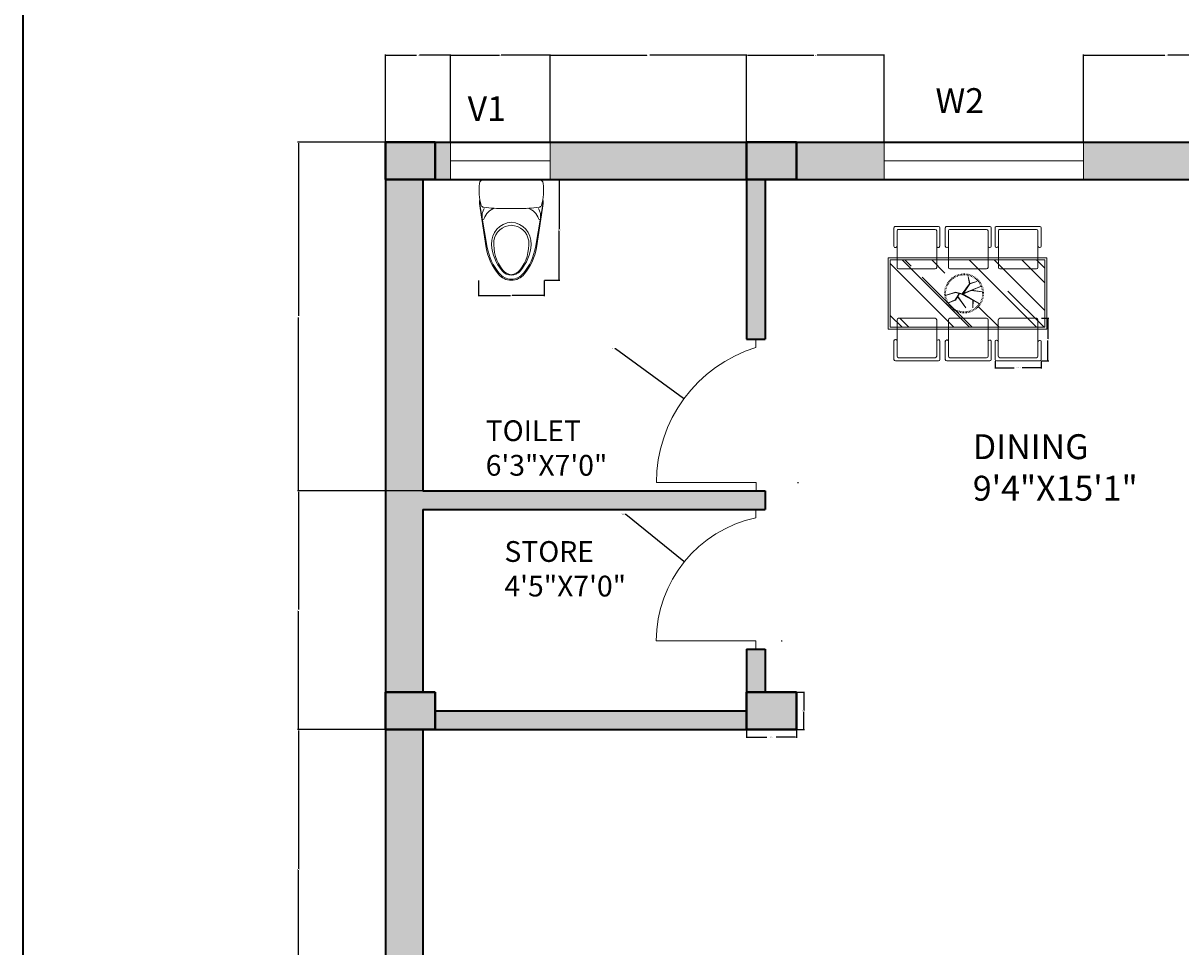
# Model space of a CAD drawing. Units: inches. Extents: x 1623 to 2200, y 2019 to 3010.
# Tile 2 of 6: x 1623 to 1902, y 2290 to 2512. Entities that reach past the tile are written whole.
import ezdxf

# ---------------------------------------------------------------- set-up
doc = ezdxf.new("R2010")
doc.units = ezdxf.units.IN
for name, color, linetype, lineweight in [('A-ANNO-DIMS', 2, 'Continuous', 18), ('A-ANNO-TTLB', 7, 'Continuous', 35), ('A-AREA-IDEN', 7, 'Continuous', 18), ('A-COLS', 7, 'Continuous', 40), ('A-DOOR', 3, 'Continuous', 18), ('A-FLOR-FIXT', 8, 'Continuous', 18), ('A-FURN', 8, 'Continuous', 13), ('A-FURN-PATT', 9, 'Continuous', 13), ('A-GLAZ', 4, 'Continuous', 18), ('A-GLAZ-IDEN', 7, 'Continuous', 18), ('A-WALL', 7, 'Continuous', 35)]:
    doc.layers.add(name, color=color, linetype=linetype, lineweight=lineweight)
doc.layers.add('A-COLS-PATT', color=152, linetype='Continuous', lineweight=13, true_color=0x2776bb)
doc.layers.add('A-WALL-PATT', color=251, linetype='Continuous', lineweight=13, true_color=0x636466)
doc.styles.get("Standard").update_dxf_attribs({"font": 'arial.ttf'})
doc.dimstyles.get("Standard").update_dxf_attribs({"dimtxt": 0.18, "dimasz": 0.18, "dimexe": 0.18, "dimexo": 0.0625, "dimgap": 0.09, "dimtad": 0, "dimtih": 1, "dimtoh": 1, "dimdec": 4, "dimzin": 0, "dimdsep": 46, "dimtxsty": 'Standard', "dimcen": 0.09, "dimadec": 0, "dimazin": 0, "dimtfac": 1, "dimtdec": 4, "dimtofl": 0, "dimtmove": 0, "dimatfit": 3, "dimfxl": 1, "dimtolj": 1, "dimtzin": 0, "dimarcsym": 0})

# ---------------------------------------------------------------- blocks, each defined once
blk = doc.blocks.new('A$C188A4A68')
at = {"ltscale": 20}
for p, q in [((0.2444, 0.7693), (0.0344, 0.7693)), ((0.2444, 0.7693), (0.4544, 0.7693)), ((0.0013, 0.5938), (0.0607, 0.2504)), ((0.0054, 0.5515), (0.0519, 0.2489)), ((0.2444, 0.5498), (0.1889, 0.5498)), ((0.2444, 0.5498), (0.2998, 0.5498)), ((0.4874, 0.5938), (0.428, 0.2504)), ((0.4833, 0.5515), (0.4368, 0.2489))]:
    blk.add_line(p, q, dxfattribs=at)
for centre, radius, start, end in [((0.442, 0.6914), 0.4447, 173.63949, 195.46404), ((0.0344, 0.7343), 0.0349, 90, 169.59261), ((0.4544, 0.7343), 0.0349, 10.40739, 90), ((0.0467, 0.6914), 0.4447, 344.53596, 6.36051), ((0.2125, 0.5932), 0.2113, 172.64979, 191.36585), ((0.2762, 0.5932), 0.2113, 348.63415, 7.35021), ((0.0333, 0.5802), 0.0213, 200.24298, 267.15028), ((0.1303, 0.4913), 0.1097, 148.50689, 190.04883), ((0.1632, 1.4554), 0.906, 261.69023, 271.62576), ((0.1461, 0.4405), 0.1134, 104.10408, 164.15012), ((0.3255, 1.4554), 0.906, 268.37424, 278.30977), ((0.3426, 0.4405), 0.1134, 15.84988, 75.89592), ((0.3584, 0.4913), 0.1097, 349.95117, 31.49311), ((0.4554, 0.5802), 0.0213, 272.84972, 339.75702), ((0.0297, 0.4734), 0.0075, 189.82636, 345.08753), ((0.254, 0.2824), 0.1613, 93.43328, 183.00378), ((0.2347, 0.2824), 0.1613, 356.99622, 86.56672), ((0.459, 0.4734), 0.0075, 194.91247, 350.17364), ((0.2493, 0.2813), 0.1393, 92.03292, 172.03731), ((0.2394, 0.2813), 0.1393, 7.96269, 87.96708), ((0.4311, 0.2946), 0.3389, 183.50421, 221.02292), ((0.4211, 0.2752), 0.3108, 175.32131, 219.24773), ((0.0676, 0.2752), 0.3108, 320.75227, 4.67869), ((0.0576, 0.2946), 0.3389, 318.97708, 356.49579), ((0.4781, 0.3243), 0.4328, 190.02971, 219.74275), ((0.4781, 0.3243), 0.4238, 190.04347, 219.7538), ((0.0106, 0.3243), 0.4238, 320.2462, 349.95653), ((0.0106, 0.3243), 0.4328, 320.25725, 349.97029), ((0.2444, 0.127), 0.127, 218.71605, 270), ((0.2444, 0.127), 0.118, 218.67741, 270), ((0.2444, 0.127), 0.088, 218.504, 270), ((0.2498, 0.1282), 0.0854, 215.56846, 266.31968), ((0.2389, 0.1282), 0.0854, 273.68032, 324.43154), ((0.2444, 0.127), 0.088, 270, 321.496), ((0.2444, 0.127), 0.118, 270, 321.32259), ((0.2444, 0.127), 0.127, 270, 321.28395)]:
    blk.add_arc(centre, radius, start, end, dxfattribs=at)
blk = doc.blocks.new('COL-12X9-PLAN')
for p, q in [((0, 0), (0, 9)), ((0, 9), (12, 9)), ((12, 9), (12, 0)), ((9, 0), (0, 0)), ((12, 0), (9, 0))]:
    blk.add_line(p, q)
blk = doc.blocks.new('WIN-48-PLAN')
for p, q in [((0, 9), (0, 0)), ((48, 4.5), (48, 9)), ((48, 9), (48, 0)), ((0, 0), (0, 4.5)), ((0, 4.5), (48, 4.5))]:
    blk.add_line(p, q)
blk = doc.blocks.new('DINING-CHAIR-FRAME')
for p, q in [((0.76, 9.92), (0.76, 1.11)), ((1.11, 10.27), (9.96, 10.27)), ((10.3, 1.11), (10.3, 9.92)), ((0, 4.79), (0, 0.34)), ((11.07, 0.34), (11.07, 4.79)), ((0.34, 0), (10.72, 0)), ((1.11, 0.76), (9.96, 0.76))]:
    blk.add_line(p, q)
for centre, start, end in [((1.11, 9.92), 90, 180), ((9.96, 9.92), 0, 90), ((0.34, 0.34), 180, 270), ((1.11, 1.11), 180, 270), ((9.96, 1.11), 270, 0), ((10.72, 0.34), 270, 0)]:
    blk.add_arc(centre, 0.343, start, end)
blk = doc.blocks.new('*D10')
at = {"layer": 'A-ANNO-DIMS', "color": 0, "lineweight": -2, "transparency": 16777216}
for p, q in [((1797.32, 2341.96), (1797.32, 2340.04)), ((1797.5, 2340.22), (1802.21, 2340.22)), ((1809.14, 2340.22), (1804.42, 2340.22)), ((1809.32, 2341.96), (1809.32, 2340.04))]:
    blk.add_line(p, q, dxfattribs=at)
at = {"layer": 'A-ANNO-DIMS', "color": 0, "transparency": 16777216}
for points in [[(1797.5, 2340.25), (1797.5, 2340.19), (1797.32, 2340.22)], [(1809.14, 2340.25), (1809.14, 2340.19), (1809.32, 2340.22)]]:
    blk.add_solid(points, dxfattribs=at)
at = {"layer": 'Defpoints', "color": 0, "transparency": 16777216}
for p in [(1797.32, 2342.02), (1809.32, 2342.02), (1809.32, 2340.22)]:
    blk.add_point(p, dxfattribs=at)
at = {"layer": 'A-ANNO-DIMS', "color": 0, "transparency": 16777216, "insert": (1803.32, 2340.22), "char_height": 0.18, "attachment_point": 5}
blk.add_mtext('\\A1;COLUMN 12 TYP.', dxfattribs=at)
blk = doc.blocks.new('*D11')
at = {"layer": 'A-ANNO-DIMS', "color": 0, "lineweight": -2, "transparency": 16777216}
for p, q in [((1809.38, 2351.02), (1811.3, 2351.02)), ((1811.12, 2350.84), (1811.12, 2346.71)), ((1811.12, 2342.2), (1811.12, 2346.34)), ((1809.38, 2342.02), (1811.3, 2342.02))]:
    blk.add_line(p, q, dxfattribs=at)
at = {"layer": 'A-ANNO-DIMS', "color": 0, "transparency": 16777216}
for points in [[(1811.09, 2350.84), (1811.15, 2350.84), (1811.12, 2351.02)], [(1811.09, 2342.2), (1811.15, 2342.2), (1811.12, 2342.02)]]:
    blk.add_solid(points, dxfattribs=at)
at = {"layer": 'Defpoints', "color": 0, "transparency": 16777216}
for p in [(1809.32, 2351.02), (1811.12, 2351.02), (1809.32, 2342.02)]:
    blk.add_point(p, dxfattribs=at)
at = {"layer": 'A-ANNO-DIMS', "color": 0, "transparency": 16777216, "insert": (1811.12, 2346.52), "char_height": 0.18, "attachment_point": 5}
blk.add_mtext('\\A1;9 TYP.', dxfattribs=at)
blk = doc.blocks.new('*D12')
at = {"layer": 'A-ANNO-DIMS', "color": 0, "lineweight": -2, "transparency": 16777216}
for p, q in [((1857.21, 2430.8), (1857.21, 2429.02)), ((1868.28, 2430.8), (1868.28, 2429.02)), ((1857.39, 2429.2), (1861.79, 2429.2)), ((1868.1, 2429.2), (1863.7, 2429.2))]:
    blk.add_line(p, q, dxfattribs=at)
at = {"layer": 'A-ANNO-DIMS', "color": 0, "transparency": 16777216}
for points in [[(1857.39, 2429.23), (1857.39, 2429.17), (1857.21, 2429.2)], [(1868.1, 2429.23), (1868.1, 2429.17), (1868.28, 2429.2)]]:
    blk.add_solid(points, dxfattribs=at)
at = {"layer": 'Defpoints', "color": 0, "transparency": 16777216}
for p in [(1857.21, 2430.86), (1868.28, 2430.86), (1868.28, 2429.2)]:
    blk.add_point(p, dxfattribs=at)
at = {"layer": 'A-ANNO-DIMS', "color": 0, "transparency": 16777216, "insert": (1862.75, 2429.2), "char_height": 0.18, "attachment_point": 5}
blk.add_mtext('\\A1;CHAIR 11 TYP.', dxfattribs=at)
blk = doc.blocks.new('*D13')
at = {"layer": 'A-ANNO-DIMS', "color": 0, "lineweight": -2, "transparency": 16777216}
for p, q in [((1868.34, 2441.13), (1870.12, 2441.13)), ((1869.94, 2440.95), (1869.94, 2436.18)), ((1869.94, 2431.04), (1869.94, 2435.81)), ((1868.34, 2430.86), (1870.12, 2430.86))]:
    blk.add_line(p, q, dxfattribs=at)
at = {"layer": 'A-ANNO-DIMS', "color": 0, "transparency": 16777216}
for points in [[(1869.91, 2440.95), (1869.97, 2440.95), (1869.94, 2441.13)], [(1869.91, 2431.04), (1869.97, 2431.04), (1869.94, 2430.86)]]:
    blk.add_solid(points, dxfattribs=at)
at = {"layer": 'Defpoints', "color": 0, "transparency": 16777216}
for p in [(1868.28, 2441.13), (1869.94, 2441.13), (1868.28, 2430.86)]:
    blk.add_point(p, dxfattribs=at)
at = {"layer": 'A-ANNO-DIMS', "color": 0, "transparency": 16777216, "insert": (1869.94, 2435.99), "char_height": 0.18, "attachment_point": 5}
blk.add_mtext('\\A1;10 TYP.', dxfattribs=at)
blk = doc.blocks.new('*D18')
at = {"layer": 'A-ANNO-DIMS', "color": 0, "lineweight": -2, "transparency": 16777216}
for p, q in [((1748.61, 2474.52), (1752.37, 2474.52)), ((1752.19, 2474.34), (1752.19, 2462.58)), ((1752.19, 2450.46), (1752.19, 2462.22)), ((1748.61, 2450.28), (1752.37, 2450.28))]:
    blk.add_line(p, q, dxfattribs=at)
at = {"layer": 'A-ANNO-DIMS', "color": 0, "transparency": 16777216}
for points in [[(1752.16, 2474.34), (1752.22, 2474.34), (1752.19, 2474.52)], [(1752.16, 2450.46), (1752.22, 2450.46), (1752.19, 2450.28)]]:
    blk.add_solid(points, dxfattribs=at)
at = {"layer": 'Defpoints', "color": 0, "transparency": 16777216}
for p in [(1748.55, 2474.52), (1752.19, 2474.52), (1748.55, 2450.28)]:
    blk.add_point(p, dxfattribs=at)
at = {"layer": 'A-ANNO-DIMS', "color": 0, "transparency": 16777216, "insert": (1752.19, 2462.4), "char_height": 0.18, "attachment_point": 5}
blk.add_mtext('\\A1;WC 24', dxfattribs=at)
blk = doc.blocks.new('*D19')
at = {"layer": 'A-ANNO-DIMS', "color": 0, "lineweight": -2, "transparency": 16777216}
for p, q in [((1732.75, 2450.21), (1732.75, 2446.46)), ((1748.55, 2450.21), (1748.55, 2446.46)), ((1732.93, 2446.64), (1740.44, 2446.64)), ((1748.37, 2446.64), (1740.86, 2446.64))]:
    blk.add_line(p, q, dxfattribs=at)
at = {"layer": 'A-ANNO-DIMS', "color": 0, "transparency": 16777216}
for points in [[(1732.93, 2446.67), (1732.93, 2446.61), (1732.75, 2446.64)], [(1748.37, 2446.67), (1748.37, 2446.61), (1748.55, 2446.64)]]:
    blk.add_solid(points, dxfattribs=at)
at = {"layer": 'Defpoints', "color": 0, "transparency": 16777216}
for p in [(1732.75, 2450.28), (1748.55, 2450.28), (1748.55, 2446.64)]:
    blk.add_point(p, dxfattribs=at)
at = {"layer": 'A-ANNO-DIMS', "color": 0, "transparency": 16777216, "insert": (1740.65, 2446.64), "char_height": 0.18, "attachment_point": 5}
blk.add_mtext('\\A1;16', dxfattribs=at)
blk = doc.blocks.new('*D30')
at = {"layer": 'A-ANNO-DIMS', "color": 0, "lineweight": -2, "transparency": 16777216}
for p, q in [((1710.33, 2483.59), (1710.33, 2504.66)), ((1725.99, 2483.59), (1725.99, 2504.66)), ((1710.51, 2504.48), (1717.77, 2504.48)), ((1725.81, 2504.48), (1718.54, 2504.48))]:
    blk.add_line(p, q, dxfattribs=at)
at = {"layer": 'A-ANNO-DIMS', "color": 0, "transparency": 16777216}
for points in [[(1710.51, 2504.51), (1710.51, 2504.45), (1710.33, 2504.48)], [(1725.81, 2504.51), (1725.81, 2504.45), (1725.99, 2504.48)]]:
    blk.add_solid(points, dxfattribs=at)
at = {"layer": 'Defpoints', "color": 0, "transparency": 16777216}
for p in [(1725.99, 2504.48), (1710.33, 2483.52), (1725.99, 2483.52)]:
    blk.add_point(p, dxfattribs=at)
at = {"layer": 'A-ANNO-DIMS', "color": 0, "transparency": 16777216, "insert": (1718.16, 2504.48), "char_height": 0.18, "attachment_point": 5}
blk.add_mtext('\\A1;15.66', dxfattribs=at)
blk = doc.blocks.new('*D31')
at = {"layer": 'A-ANNO-DIMS', "color": 0, "lineweight": -2, "transparency": 16777216}
for p, q in [((1725.99, 2483.59), (1725.99, 2504.66)), ((1749.99, 2483.59), (1749.99, 2504.66)), ((1726.17, 2504.48), (1737.77, 2504.48)), ((1749.81, 2504.48), (1738.21, 2504.48))]:
    blk.add_line(p, q, dxfattribs=at)
at = {"layer": 'A-ANNO-DIMS', "color": 0, "transparency": 16777216}
for points in [[(1726.17, 2504.51), (1726.17, 2504.45), (1725.99, 2504.48)], [(1749.81, 2504.51), (1749.81, 2504.45), (1749.99, 2504.48)]]:
    blk.add_solid(points, dxfattribs=at)
at = {"layer": 'Defpoints', "color": 0, "transparency": 16777216}
for p in [(1749.99, 2504.48), (1725.99, 2483.52), (1749.99, 2483.52)]:
    blk.add_point(p, dxfattribs=at)
at = {"layer": 'A-ANNO-DIMS', "color": 0, "transparency": 16777216, "insert": (1737.99, 2504.48), "char_height": 0.18, "attachment_point": 5}
blk.add_mtext('\\A1;24', dxfattribs=at)
blk = doc.blocks.new('*D32')
at = {"layer": 'A-ANNO-DIMS', "color": 0, "lineweight": -2, "transparency": 16777216}
for p, q in [((1749.99, 2483.59), (1749.99, 2504.66)), ((1797.33, 2483.59), (1797.33, 2504.66)), ((1750.17, 2504.48), (1773.26, 2504.48)), ((1797.15, 2504.48), (1774.05, 2504.48))]:
    blk.add_line(p, q, dxfattribs=at)
at = {"layer": 'A-ANNO-DIMS', "color": 0, "transparency": 16777216}
for points in [[(1750.17, 2504.51), (1750.17, 2504.45), (1749.99, 2504.48)], [(1797.15, 2504.51), (1797.15, 2504.45), (1797.33, 2504.48)]]:
    blk.add_solid(points, dxfattribs=at)
at = {"layer": 'Defpoints', "color": 0, "transparency": 16777216}
for p in [(1797.33, 2504.48), (1749.99, 2483.52), (1797.33, 2483.52)]:
    blk.add_point(p, dxfattribs=at)
at = {"layer": 'A-ANNO-DIMS', "color": 0, "transparency": 16777216, "insert": (1773.66, 2504.48), "char_height": 0.18, "attachment_point": 5}
blk.add_mtext('\\A1;47.34', dxfattribs=at)
blk = doc.blocks.new('*D33')
at = {"layer": 'A-ANNO-DIMS', "color": 0, "lineweight": -2, "transparency": 16777216}
for p, q in [((1797.33, 2483.59), (1797.33, 2504.66)), ((1830.5, 2483.59), (1830.5, 2504.66)), ((1797.51, 2504.48), (1813.52, 2504.48)), ((1830.32, 2504.48), (1814.31, 2504.48))]:
    blk.add_line(p, q, dxfattribs=at)
at = {"layer": 'A-ANNO-DIMS', "color": 0, "transparency": 16777216}
for points in [[(1797.51, 2504.51), (1797.51, 2504.45), (1797.33, 2504.48)], [(1830.32, 2504.51), (1830.32, 2504.45), (1830.5, 2504.48)]]:
    blk.add_solid(points, dxfattribs=at)
at = {"layer": 'Defpoints', "color": 0, "transparency": 16777216}
for p in [(1830.5, 2504.48), (1797.33, 2483.52), (1830.5, 2483.52)]:
    blk.add_point(p, dxfattribs=at)
at = {"layer": 'A-ANNO-DIMS', "color": 0, "transparency": 16777216, "insert": (1813.91, 2504.48), "char_height": 0.18, "attachment_point": 5}
blk.add_mtext('\\A1;33.17', dxfattribs=at)
blk = doc.blocks.new('*D34')
at = {"layer": 'A-ANNO-DIMS', "color": 0, "lineweight": -2, "transparency": 16777216}
for p, q in [((1878.5, 2483.59), (1878.5, 2504.66)), ((1918.4, 2483.59), (1918.4, 2504.66)), ((1878.68, 2504.48), (1898.12, 2504.48)), ((1918.22, 2504.48), (1898.77, 2504.48))]:
    blk.add_line(p, q, dxfattribs=at)
at = {"layer": 'A-ANNO-DIMS', "color": 0, "transparency": 16777216}
for points in [[(1878.68, 2504.51), (1878.68, 2504.45), (1878.5, 2504.48)], [(1918.22, 2504.51), (1918.22, 2504.45), (1918.4, 2504.48)]]:
    blk.add_solid(points, dxfattribs=at)
at = {"layer": 'Defpoints', "color": 0, "transparency": 16777216}
for p in [(1918.4, 2504.48), (1878.5, 2483.52), (1918.4, 2483.52)]:
    blk.add_point(p, dxfattribs=at)
at = {"layer": 'A-ANNO-DIMS', "color": 0, "transparency": 16777216, "insert": (1898.45, 2504.48), "char_height": 0.18, "attachment_point": 5}
blk.add_mtext('\\A1;39.9', dxfattribs=at)
blk = doc.blocks.new('*D41')
at = {"layer": 'A-ANNO-DIMS', "color": 0, "lineweight": -2, "transparency": 16777216}
for p, q in [((1710.26, 2342.02), (1689.17, 2342.02)), ((1689.35, 2341.84), (1689.35, 2308.49)), ((1689.35, 2274.77), (1689.35, 2308.13)), ((1719.26, 2274.59), (1689.17, 2274.59))]:
    blk.add_line(p, q, dxfattribs=at)
at = {"layer": 'A-ANNO-DIMS', "color": 0, "transparency": 16777216}
for points in [[(1689.32, 2341.84), (1689.38, 2341.84), (1689.35, 2342.02)], [(1689.32, 2274.77), (1689.38, 2274.77), (1689.35, 2274.59)]]:
    blk.add_solid(points, dxfattribs=at)
at = {"layer": 'Defpoints', "color": 0, "transparency": 16777216}
for p in [(1689.35, 2342.02), (1710.32, 2342.02), (1719.33, 2274.59)]:
    blk.add_point(p, dxfattribs=at)
at = {"layer": 'A-ANNO-DIMS', "color": 0, "transparency": 16777216, "insert": (1689.35, 2308.31), "char_height": 0.18, "attachment_point": 5}
blk.add_mtext('\\A1;67.43', dxfattribs=at)
blk = doc.blocks.new('*D42')
at = {"layer": 'A-ANNO-DIMS', "color": 0, "lineweight": -2, "transparency": 16777216}
for p, q in [((1719.26, 2399.52), (1689.17, 2399.52)), ((1689.35, 2399.34), (1689.35, 2370.96)), ((1689.35, 2342.2), (1689.35, 2370.59)), ((1710.26, 2342.02), (1689.17, 2342.02))]:
    blk.add_line(p, q, dxfattribs=at)
at = {"layer": 'A-ANNO-DIMS', "color": 0, "transparency": 16777216}
for points in [[(1689.32, 2399.34), (1689.38, 2399.34), (1689.35, 2399.52)], [(1689.32, 2342.2), (1689.38, 2342.2), (1689.35, 2342.02)]]:
    blk.add_solid(points, dxfattribs=at)
at = {"layer": 'Defpoints', "color": 0, "transparency": 16777216}
for p in [(1689.35, 2399.52), (1719.33, 2399.52), (1710.32, 2342.02)]:
    blk.add_point(p, dxfattribs=at)
at = {"layer": 'A-ANNO-DIMS', "color": 0, "transparency": 16777216, "insert": (1689.35, 2370.77), "char_height": 0.18, "attachment_point": 5}
blk.add_mtext('\\A1;57.5', dxfattribs=at)
blk = doc.blocks.new('*D43')
at = {"layer": 'A-ANNO-DIMS', "color": 0, "lineweight": -2, "transparency": 16777216}
for p, q in [((1710.26, 2483.52), (1689.17, 2483.52)), ((1689.35, 2483.34), (1689.35, 2441.71)), ((1689.35, 2399.7), (1689.35, 2441.34)), ((1719.26, 2399.52), (1689.17, 2399.52))]:
    blk.add_line(p, q, dxfattribs=at)
at = {"layer": 'A-ANNO-DIMS', "color": 0, "transparency": 16777216}
for points in [[(1689.32, 2483.34), (1689.38, 2483.34), (1689.35, 2483.52)], [(1689.32, 2399.7), (1689.38, 2399.7), (1689.35, 2399.52)]]:
    blk.add_solid(points, dxfattribs=at)
at = {"layer": 'Defpoints', "color": 0, "transparency": 16777216}
for p in [(1689.35, 2483.52), (1710.33, 2483.52), (1719.33, 2399.52)]:
    blk.add_point(p, dxfattribs=at)
at = {"layer": 'A-ANNO-DIMS', "color": 0, "transparency": 16777216, "insert": (1689.35, 2441.52), "char_height": 0.18, "attachment_point": 5}
blk.add_mtext('\\A1;84', dxfattribs=at)
blk = doc.blocks.new('*D61')
at = {"layer": 'A-ANNO-DIMS', "color": 0, "lineweight": -2, "transparency": 16777216}
for p, q in [((1765.58, 2433.87), (1765.76, 2433.87)), ((1765.76, 2433.87), (1782.1, 2421.85)), ((1809.64, 2401.52), (1809.82, 2401.52)), ((1809.73, 2401.43), (1809.73, 2401.61))]:
    blk.add_line(p, q, dxfattribs=at)
at = {"layer": 'A-ANNO-DIMS', "color": 0, "transparency": 16777216}
blk.add_solid([(1782.12, 2421.87), (1782.09, 2421.82), (1782.25, 2421.74)], dxfattribs=at)
at = {"layer": 'Defpoints', "color": 0, "transparency": 16777216}
for p in [(1782.25, 2421.74), (1809.73, 2401.52)]:
    blk.add_point(p, dxfattribs=at)
at = {"layer": 'A-ANNO-DIMS', "color": 0, "transparency": 16777216, "insert": (1765.1, 2433.87), "char_height": 0.18, "attachment_point": 5}
blk.add_mtext('\\A1;R34.12', dxfattribs=at)
blk = doc.blocks.new('*D62')
at = {"layer": 'A-ANNO-DIMS', "color": 0, "lineweight": -2, "transparency": 16777216}
for p, q in [((1768.06, 2393.92), (1768.24, 2393.92)), ((1768.24, 2393.92), (1782.19, 2382.6)), ((1805.72, 2363.44), (1805.9, 2363.44)), ((1805.81, 2363.35), (1805.81, 2363.53))]:
    blk.add_line(p, q, dxfattribs=at)
at = {"layer": 'A-ANNO-DIMS', "color": 0, "transparency": 16777216}
blk.add_solid([(1782.21, 2382.63), (1782.17, 2382.58), (1782.33, 2382.49)], dxfattribs=at)
at = {"layer": 'Defpoints', "color": 0, "transparency": 16777216}
for p in [(1782.33, 2382.49), (1805.81, 2363.44)]:
    blk.add_point(p, dxfattribs=at)
at = {"layer": 'A-ANNO-DIMS', "color": 0, "transparency": 16777216, "insert": (1767.59, 2393.92), "char_height": 0.18, "attachment_point": 5}
blk.add_mtext('\\A1;R30.23', dxfattribs=at)

msp = doc.modelspace()

# ---------------------------------------------------------------- hatches: boundary and pattern name
at = {"layer": 'A-COLS-PATT'}
h = msp.add_hatch(color=256, dxfattribs=at)
h.dxf.hatch_style = 1
h.paths.add_polyline_path([(1722.3258, 2483.5237), (1710.3258, 2483.5237), (1710.3258, 2474.5237), (1719.3258, 2474.5237), (1722.3258, 2474.5237)])
h.paths.add_polyline_path([(1809.3258, 2483.5237), (1797.3258, 2483.5237), (1797.3258, 2474.5237), (1806.3258, 2474.5237), (1809.3258, 2474.5237)])
h.paths.add_polyline_path([(1918.3972, 2483.5237), (1906.3972, 2483.5237), (1906.3972, 2474.5237), (1915.3972, 2474.5237), (1918.3972, 2474.5237)])
h.paths.add_polyline_path([(2071.3258, 2483.5237), (2059.3258, 2483.5237), (2059.3258, 2474.532), (2068.3258, 2474.532), (2071.3258, 2474.532)])
h.paths.add_polyline_path([(2071.3258, 2351.0312), (2059.3258, 2351.0312), (2059.3258, 2342.0312), (2068.3258, 2342.0312), (2071.3258, 2342.0312)])
h.paths.add_polyline_path([(1918.3258, 2351.0237), (1906.3258, 2351.0237), (1906.3258, 2342.0237), (1915.3258, 2342.0237), (1918.3258, 2342.0237)])
h.paths.add_polyline_path([(1722.3198, 2351.0237), (1710.3258, 2351.0237), (1710.3258, 2342.0237), (1719.3198, 2342.0237), (1722.3198, 2342.0237)])
h.paths.add_polyline_path([(1809.3158, 2351.0237), (1797.3258, 2351.0237), (1797.3258, 2346.5237), (1797.3158, 2342.0237), (1806.3158, 2342.0237), (1809.3158, 2342.0237)])
h.paths.add_polyline_path([(1722.3029, 2170.0237), (1710.3258, 2170.0237), (1710.3258, 2161.0237), (1714.3029, 2161.0237), (1719.3029, 2161.0237), (1722.3029, 2161.0237)])
h.paths.add_polyline_path([(1809.3258, 2170.0237), (1797.3258, 2170.0237), (1797.3258, 2161.0237), (1801.3258, 2161.0237), (1802.9141, 2161.0237), (1806.3258, 2161.0237), (1809.3258, 2161.0237)])
h.paths.add_polyline_path([(1918.2273, 2170.0237), (1906.2273, 2170.0237), (1906.2273, 2161.0237), (1915.2273, 2161.0237), (1918.2273, 2161.0237)])
h.paths.add_polyline_path([(2071.3258, 2170.0237), (2059.3258, 2170.0237), (2059.3258, 2161.0237), (2068.3258, 2161.0237), (2071.3258, 2161.0237)])
at = {"layer": 'A-FURN-PATT'}
h = msp.add_hatch(dxfattribs=at)
h.set_pattern_fill('AR-RROOF', color=256, scale=11.449163, angle=-45, style=0)
h.set_pattern_definition([(315, (2208.266, 3409.365), (25.9065, -9.71494), [171.7375, -22.8983, 57.2458, -11.4492]), (315, (2223.081, 3402.646), (2.6716, 18.86317), [34.3475, -3.7782, 68.695, -8.5869]), (315, (2219.195, 3412.199), (47.522235, -36.67389), [91.5933, -16.02883, 45.79665, -11.44916])])
h.paths.add_polyline_path([(1831.9482, 2438.9568), (1869.158, 2438.9568), (1869.158, 2455.1764), (1831.9482, 2455.1764)])
at = {"layer": 'A-WALL-PATT'}
h = msp.add_hatch(color=256, dxfattribs=at)
h.dxf.hatch_style = 1
h.paths.add_polyline_path([(1725.9857, 2483.5237), (1722.3258, 2483.5237), (1722.3258, 2474.5237), (1725.9857, 2474.5237), (1725.9857, 2479.0237)])
h.paths.add_polyline_path([(1797.3258, 2483.5237), (1749.9857, 2483.5237), (1749.9857, 2474.5237), (1797.3258, 2474.5237)])
h.paths.add_polyline_path([(1830.4977, 2483.5237), (1809.3258, 2483.5237), (1809.3258, 2474.5237), (1830.4977, 2474.5237), (1830.4977, 2479.0237)])
h.paths.add_polyline_path([(1906.3972, 2483.5237), (1878.4977, 2483.5237), (1878.4977, 2474.5237), (1906.3972, 2474.5237)])
h.paths.add_polyline_path([(1918.3258, 2474.5237), (1915.3972, 2474.5237), (1913.8258, 2474.5237), (1913.8258, 2395.0237), (1913.8258, 2384.7587), (1918.3258, 2384.7587), (1918.3258, 2395.0237)])
h.paths.add_polyline_path([(1801.8258, 2474.5237), (1797.3258, 2474.5237), (1797.3258, 2436.0951), (1801.8258, 2436.0951)], flags=17)
h.paths.add_polyline_path([(1719.3258, 2474.5237), (1710.3258, 2474.5237), (1710.3258, 2351.0237), (1719.3258, 2351.0237), (1719.3258, 2395.0237), (1801.8258, 2395.0237), (1801.8258, 2399.5237), (1719.3258, 2399.5237)])
h.paths.add_polyline_path([(1797.3158, 2346.5237), (1722.3198, 2346.5237), (1722.3198, 2342.0237), (1797.3158, 2342.0237)])
h.paths.add_polyline_path([(1801.8258, 2361.4421), (1797.3258, 2361.4421), (1797.3258, 2351.0237), (1801.8258, 2351.0237)], flags=17)
h.paths.add_polyline_path([(2059.3258, 2346.5237), (1918.3258, 2346.5237), (1918.3258, 2342.0237), (2059.3258, 2342.0237)])
h.paths.add_polyline_path([(1963.26, 2479.0237), (1963.26, 2483.5237), (1918.3972, 2483.5237), (1918.3972, 2474.5237), (1963.26, 2474.5237)])
h.paths.add_polyline_path([(2059.3258, 2483.5237), (2011.26, 2483.5237), (2011.26, 2474.5237), (2059.3258, 2474.5237)])
h.paths.add_polyline_path([(2071.3258, 2474.532), (2068.3258, 2474.532), (2062.3258, 2474.532), (2062.3258, 2351.0312), (2071.3258, 2351.0312)])
h.paths.add_polyline_path([(2071.3258, 2342.0312), (2068.3258, 2342.0312), (2062.3258, 2342.0312), (2062.3258, 2170.0237), (2071.3258, 2170.0237)])
h.paths.add_polyline_path([(2059.3258, 2170.0237), (2038.3258, 2170.0237), (2038.3258, 2161.0237), (2059.3258, 2161.0237)])
h.paths.add_polyline_path([(1990.3258, 2170.0237), (1963.4402, 2170.0237), (1963.4402, 2161.0237), (1990.3258, 2161.0237), (1990.3258, 2165.5237)])
h.paths.add_polyline_path([(1918.3258, 2274.595), (1913.8258, 2274.595), (1913.8258, 2170.0237), (1918.3258, 2170.0237)])
h.paths.add_polyline_path([(1906.2273, 2170.0237), (1871.454, 2170.0237), (1871.454, 2161.0237), (1906.2273, 2161.0237)])
h.paths.add_polyline_path([(1835.454, 2170.0237), (1809.3258, 2170.0237), (1809.3258, 2161.0237), (1835.454, 2161.0237), (1835.454, 2165.5237)])
h.paths.add_polyline_path([(1801.8258, 2270.095), (1865.2406, 2270.095), (1865.2406, 2274.595), (1797.3258, 2274.595), (1797.3258, 2170.0237), (1801.8258, 2170.0237)])
h.paths.add_polyline_path([(1719.3258, 2342.0237), (1719.3198, 2342.0237), (1710.3258, 2342.0237), (1710.3258, 2170.0237), (1719.3258, 2170.0237)])

# ---------------------------------------------------------------- linework, layer by layer
at = {"layer": 'A-ANNO-TTLB'}
msp.add_lwpolyline([(1623.0453, 3010.4913), (2200.0052, 3010.4913), (2200.0052, 2019.4245), (1623.0453, 2019.4245)], close=True, dxfattribs=at)
at = {"layer": 'A-DOOR'}
for p, q in [((1799.5758, 2436.0951), (1799.5758, 2434.0951)), ((1799.6124, 2401.5237), (1775.6124, 2401.5237)), ((1799.6124, 2399.5237), (1799.6124, 2401.5237)), ((1799.5758, 2395.0237), (1799.5758, 2393.0237)), ((1799.5758, 2363.4421), (1775.5758, 2363.4421)), ((1799.5758, 2361.4421), (1799.5758, 2363.4421))]:
    msp.add_line(p, q, dxfattribs=at)
for centre, radius, start in [((1809.7299, 2401.5237), 34.1175, 107.314846), ((1805.8064, 2363.4421), 30.2306, 101.894118)]:
    msp.add_arc(centre, radius, start, 180, dxfattribs=at)
at = {"layer": 'A-FURN'}
for p, q in [((1833.1681, 2458.1396), (1833.2445, 2458.1396)), ((1843.4724, 2458.1396), (1843.5487, 2458.1396)), ((1845.5473, 2458.1396), (1845.6236, 2458.1396)), ((1855.8515, 2458.1396), (1855.9279, 2458.1396)), ((1857.6337, 2458.1396), (1857.5574, 2458.1396)), ((1867.938, 2458.1396), (1867.8617, 2458.1396)), ((1869.635, 2455.6535), (1831.4711, 2455.6535)), ((1831.4711, 2455.6535), (1831.4711, 2438.4797)), ((1869.158, 2455.1764), (1831.9482, 2455.1764)), ((1831.9482, 2455.1764), (1831.9482, 2438.9568)), ((1869.158, 2438.9568), (1869.158, 2455.1764)), ((1869.635, 2438.4797), (1869.635, 2455.6535)), ((1848.1587, 2451.2177), (1848.0223, 2451.5741)), ((1848.4851, 2451.3281), (1848.3771, 2451.6941)), ((1848.8192, 2451.4126), (1848.7403, 2451.7859)), ((1849.1589, 2451.4705), (1849.1095, 2451.849)), ((1849.5021, 2451.5017), (1849.4826, 2451.8828)), ((1849.8467, 2451.5058), (1849.8571, 2451.8873)), ((1850.1905, 2451.4829), (1850.2308, 2451.8624)), ((1850.5315, 2451.4331), (1850.6015, 2451.8083)), ((1850.8676, 2451.3567), (1850.9667, 2451.7252)), ((1851.1966, 2451.2541), (1851.3243, 2451.6137)), ((1845.7196, 2448.9081), (1845.3711, 2449.0637)), ((1845.8723, 2449.217), (1845.5371, 2449.3995)), ((1846.0488, 2449.513), (1845.729, 2449.7212)), ((1846.248, 2449.7942), (1845.9455, 2450.0268)), ((1846.4687, 2450.0589), (1846.1853, 2450.3146)), ((1846.7094, 2450.3055), (1846.447, 2450.5826)), ((1846.9688, 2450.5324), (1846.7289, 2450.8293)), ((1847.2451, 2450.7383), (1847.0293, 2451.0531)), ((1847.5367, 2450.9219), (1847.3463, 2451.2526)), ((1847.8419, 2451.082), (1847.678, 2451.4266)), ((1851.0336, 2449.4046), (1849.2274, 2447.0176)), ((1853.8962, 2448.859), (1849.2274, 2447.0176)), ((1849.466, 2447.0517), (1851.1358, 2449.4046)), ((1850.7269, 2451.1779), (1851.0336, 2449.4046)), ((1851.1018, 2449.4728), (1850.7269, 2451.1779)), ((1852.8057, 2450.0185), (1851.1018, 2449.4728)), ((1851.1358, 2449.4046), (1852.8057, 2450.0185)), ((1851.5165, 2451.1261), (1851.6721, 2451.4746)), ((1851.6225, 2447.869), (1853.8962, 2448.859)), ((1851.8254, 2450.9733), (1852.0079, 2451.3085)), ((1852.1214, 2450.7968), (1852.3296, 2451.1167)), ((1852.4026, 2450.5976), (1852.6352, 2450.9001)), ((1852.6673, 2450.377), (1852.923, 2450.6603)), ((1852.9139, 2450.1362), (1853.191, 2450.3986)), ((1853.1408, 2449.8769), (1853.4377, 2450.1168)), ((1853.3467, 2449.6006), (1853.6615, 2449.8164)), ((1853.5303, 2449.3089), (1853.861, 2449.4994)), ((1853.6904, 2449.0038), (1854.035, 2449.1677)), ((1853.8261, 2448.687), (1854.1825, 2448.8234)), ((1845.3398, 2447.2383), (1844.9583, 2447.2487)), ((1845.344, 2446.8937), (1844.9628, 2446.8741)), ((1845.3627, 2447.5821), (1844.9832, 2447.6224)), ((1845.3751, 2446.5505), (1844.9967, 2446.5011)), ((1845.4125, 2447.9231), (1845.0374, 2447.9931)), ((1845.4331, 2446.2108), (1845.0597, 2446.1319)), ((1845.489, 2448.2592), (1845.1204, 2448.3583)), ((1847.6258, 2447.4268), (1845.2062, 2446.5742)), ((1845.2062, 2446.5742), (1847.6258, 2447.3245)), ((1845.5915, 2448.5882), (1845.2319, 2448.7159)), ((1848.614, 2447.1881), (1847.5917, 2445.5853)), ((1849.2274, 2447.0517), (1847.6258, 2447.4268)), ((1847.6258, 2447.3245), (1849.4319, 2446.8812)), ((1847.6939, 2445.5171), (1848.6481, 2447.0858)), ((1850.1476, 2443.6416), (1848.1369, 2446.3355)), ((1848.2392, 2446.3355), (1850.1476, 2443.6416)), ((1851.8515, 2445.4694), (1849.2615, 2446.8812)), ((1849.4319, 2446.9153), (1851.4446, 2447.7916)), ((1849.466, 2446.9153), (1853.4532, 2444.5964)), ((1854.0666, 2447.495), (1851.4446, 2447.7916)), ((1851.6225, 2447.869), (1854.0666, 2447.495)), ((1853.9365, 2448.3605), (1854.3025, 2448.4685)), ((1853.9651, 2445.9781), (1854.3336, 2445.8789)), ((1854.021, 2448.0264), (1854.3943, 2448.1054)), ((1854.0415, 2446.3141), (1854.4167, 2446.2442)), ((1854.079, 2447.6867), (1854.4574, 2447.7361)), ((1854.0913, 2446.6551), (1854.4708, 2446.6148)), ((1854.1101, 2447.3435), (1854.4912, 2447.3631)), ((1854.1142, 2446.999), (1854.4957, 2446.9886)), ((1845.5176, 2445.8767), (1845.1515, 2445.7687)), ((1845.628, 2445.5503), (1845.2715, 2445.4139)), ((1845.7637, 2445.2335), (1845.419, 2445.0696)), ((1845.9238, 2444.9283), (1845.5931, 2444.7379)), ((1846.1074, 2444.6367), (1845.7926, 2444.4209)), ((1847.5917, 2445.5853), (1845.9559, 2444.8351)), ((1845.9559, 2444.8351), (1847.6939, 2445.5171)), ((1846.3133, 2444.3604), (1846.0164, 2444.1205)), ((1846.5402, 2444.101), (1846.2631, 2443.8386)), ((1846.7868, 2443.8603), (1846.5311, 2443.5769)), ((1847.0515, 2443.6396), (1846.8188, 2443.3371)), ((1847.3327, 2443.4404), (1847.1245, 2443.1206)), ((1847.6287, 2443.2639), (1847.4462, 2442.9287)), ((1851.6122, 2443.1553), (1851.7761, 2442.8106)), ((1851.8515, 2443.6075), (1851.8515, 2445.4694)), ((1851.9316, 2445.4257), (1851.8515, 2443.6075)), ((1851.9173, 2443.3154), (1852.1078, 2442.9847)), ((1853.4532, 2444.5964), (1851.9316, 2445.4257)), ((1852.209, 2443.499), (1852.4248, 2443.1842)), ((1852.4853, 2443.7048), (1852.7252, 2443.408)), ((1852.7446, 2443.9318), (1853.007, 2443.6547)), ((1852.9854, 2444.1784), (1853.2687, 2443.9227)), ((1853.206, 2444.4431), (1853.5085, 2444.2104)), ((1853.4052, 2444.7243), (1853.7251, 2444.5161)), ((1853.5817, 2445.0203), (1853.9169, 2444.8378)), ((1853.7345, 2445.3292), (1854.083, 2445.1736)), ((1853.8625, 2445.6491), (1854.2222, 2445.5213)), ((1847.9376, 2443.1112), (1847.782, 2442.7627)), ((1848.2575, 2442.9831), (1848.1297, 2442.6235)), ((1848.5865, 2442.8806), (1848.4873, 2442.512)), ((1848.9225, 2442.8041), (1848.8526, 2442.429)), ((1849.2635, 2442.7543), (1849.2232, 2442.3748)), ((1849.6074, 2442.7314), (1849.597, 2442.3499)), ((1849.952, 2442.7355), (1849.9715, 2442.3544)), ((1850.2951, 2442.7667), (1850.3446, 2442.3883)), ((1850.6348, 2442.8247), (1850.7138, 2442.4513)), ((1850.9689, 2442.9092), (1851.0769, 2442.5431)), ((1851.2954, 2443.0196), (1851.4318, 2442.6631)), ((1831.4711, 2438.4797), (1869.635, 2438.4797)), ((1831.9482, 2438.9568), (1869.158, 2438.9568)), ((1833.1704, 2435.9914), (1833.2467, 2435.9909)), ((1843.4744, 2435.9231), (1843.5508, 2435.9226)), ((1845.5493, 2435.9093), (1845.6256, 2435.9088)), ((1855.8533, 2435.841), (1855.9296, 2435.8405)), ((1857.6355, 2435.8292), (1857.5592, 2435.8297)), ((1867.9395, 2435.7609), (1867.8632, 2435.7614))]:
    msp.add_line(p, q, dxfattribs=at)
for centre, start, end in [((1833.1681, 2458.483), 180, 0.103974), ((1843.4724, 2458.483), 180, 0.103974), ((1845.5473, 2458.483), 180, 270), ((1845.6236, 2458.483), 270, 0), ((1855.8515, 2458.483), 180, 270), ((1855.9279, 2458.483), 270, 0), ((1857.5574, 2458.483), 180, 270), ((1857.6337, 2458.483), 270, 0), ((1867.8617, 2458.483), 180, 270), ((1867.938, 2458.483), 270, 0), ((1833.1681, 2435.6479), 89.620247, 179.620246), ((1833.2445, 2435.6474), 359.620246, 89.620247), ((1843.4722, 2435.5796), 89.620247, 179.620246), ((1843.5485, 2435.5791), 359.620246, 89.620247), ((1845.547, 2435.5659), 89.620247, 179.620246), ((1845.6233, 2435.5653), 359.620246, 89.620247), ((1855.851, 2435.4976), 89.620247, 179.620246), ((1855.9273, 2435.497), 359.620246, 89.620247), ((1857.5569, 2435.4862), 89.620247, 179.620246), ((1857.6332, 2435.4857), 359.620246, 89.620247), ((1867.8609, 2435.418), 89.620247, 179.620246), ((1867.9372, 2435.4174), 359.620246, 89.620247)]:
    msp.add_arc(centre, 0.3435, start, end, dxfattribs=at)
at = {"layer": 'A-GLAZ'}
for p, q in [((1725.9857, 2483.5237), (1725.9857, 2474.5237)), ((1749.9857, 2479.0237), (1749.9857, 2483.5237)), ((1749.9857, 2483.5237), (1749.9857, 2474.5237)), ((1725.9857, 2474.5237), (1725.9857, 2479.0237)), ((1725.9857, 2479.0237), (1749.9857, 2479.0237))]:
    msp.add_line(p, q, dxfattribs=at)
at = {"layer": 'A-WALL'}
for p, q in [((1710.3258, 2483.5237), (2071.3258, 2483.5237)), ((1710.3258, 2483.5237), (1710.3258, 2161.0237)), ((1719.3258, 2474.5237), (1797.3258, 2474.5237)), ((1719.3258, 2474.5237), (1719.3258, 2399.5237)), ((1797.3258, 2474.5237), (1797.3258, 2436.0951)), ((1801.8258, 2474.5237), (1801.8258, 2436.0951)), ((1801.8258, 2474.5237), (1913.8258, 2474.5237)), ((1797.3258, 2436.0951), (1801.8258, 2436.0951)), ((1719.3258, 2399.5237), (1801.8258, 2399.5237)), ((1801.8258, 2399.5237), (1801.8258, 2395.0237)), ((1719.3258, 2395.0237), (1801.8258, 2395.0237)), ((1719.3258, 2395.0237), (1719.3258, 2351.0237)), ((1797.3258, 2361.4421), (1801.8258, 2361.4421)), ((1797.3258, 2361.4421), (1797.3258, 2346.5237)), ((1801.8258, 2361.4421), (1801.8258, 2351.0237)), ((1722.3198, 2346.5237), (1797.3258, 2346.5237)), ((1719.3258, 2342.0237), (1801.8258, 2342.0237)), ((1719.3258, 2342.0237), (1719.3258, 2170.0237))]:
    msp.add_line(p, q, dxfattribs=at)

# ---------------------------------------------------------------- block references
at = {"layer": 'A-COLS'}
for p in [(1710.326, 2474.524), (1797.326, 2474.524), (1710.32, 2342.024), (1797.3161, 2342.024)]:
    msp.add_blockref('COL-12X9-PLAN', p, dxfattribs=at)
at = {"layer": 'A-FLOR-FIXT', "xscale": 31.52005674060135, "yscale": 31.52005674060135, "zscale": 31.52005674060135}
msp.add_blockref('A$C188A4A68', (1732.9465, 2450.2767), dxfattribs=at)
at = {"layer": 'A-FURN', "rotation": 180}
for p in [(1843.8919, 2463.2732), (1856.271, 2463.2732), (1868.2811, 2463.2732)]:
    msp.add_blockref('DINING-CHAIR-FRAME', p, dxfattribs=at)
at = {"layer": 'A-FURN'}
for p in [(1832.825, 2430.86), (1845.2041, 2430.86), (1857.2143, 2430.86)]:
    msp.add_blockref('DINING-CHAIR-FRAME', p, dxfattribs=at)
at = {"layer": 'A-GLAZ'}
msp.add_blockref('WIN-48-PLAN', (1830.498, 2474.524), dxfattribs=at)

# ---------------------------------------------------------------- texts
at = {"layer": 'A-AREA-IDEN', "attachment_point": 1}
for s, width, insert, char_height in [('TOILET\\P6\'3"X7\'0"', 125.471625, (1734.4771, 2416.5299), 5), ('DINING \\P9\'4"X15\'1"', 129.201541, (1851.8279, 2413.1838), 6), ('STORE\\P4\'5"X7\'0"', 68.530209, (1738.9886, 2387.4326), 5)]:
    msp.add_mtext_dynamic_manual_height_columns(s, width=width, gutter_width=12.5, heights=[0], dxfattribs=dict(at, insert=insert, char_height=char_height))
at = {"layer": 'A-GLAZ-IDEN', "char_height": 6, "attachment_point": 1}
for s, width, insert in [('W2', 54.397259, (1842.823, 2496.5633)), ('V1', 51.079224, (1730.1182, 2494.6363))]:
    msp.add_mtext_dynamic_manual_height_columns(s, width=width, gutter_width=12.5, heights=[0], dxfattribs=dict(at, insert=insert))

# ---------------------------------------------------------------- dimensions: what is measured, and where the dimension line sits
at = {"layer": 'A-ANNO-DIMS'}
for base, p1, p2, override, picture, middle in [((1725.9857, 2504.482), (1710.3258, 2483.5237), (1725.9857, 2483.5237), {"dimdec": 2, "dimlfac": 1, "dimrnd": 0, "dimzin": 0, "dimdsep": 46, "dimlunit": 2}, '*D30', (1718.1557, 2504.482)), ((1749.9857, 2504.482), (1725.9857, 2483.5237), (1749.9857, 2483.5237), {"dimdec": 0, "dimlfac": 1, "dimrnd": 0, "dimzin": 0, "dimdsep": 46, "dimlunit": 2}, '*D31', (1737.9857, 2504.482)), ((1797.3258, 2504.482), (1749.9857, 2483.5237), (1797.3258, 2483.5237), {"dimdec": 2, "dimlfac": 1, "dimrnd": 0, "dimzin": 0, "dimdsep": 46, "dimlunit": 2}, '*D32', (1773.6557, 2504.482)), ((1830.4977, 2504.482), (1797.3258, 2483.5237), (1830.4977, 2483.5237), {"dimdec": 2, "dimlfac": 1, "dimrnd": 0, "dimzin": 0, "dimdsep": 46, "dimlunit": 2}, '*D33', (1813.9118, 2504.482)), ((1918.3972, 2504.482), (1878.4977, 2483.5237), (1918.3972, 2483.5237), {"dimdec": 1, "dimlfac": 1, "dimrnd": 0, "dimzin": 0, "dimdsep": 46, "dimlunit": 2}, '*D34', (1898.4475, 2504.482)), ((1748.5482, 2446.6397), (1732.7488, 2450.2767), (1748.5482, 2450.2767), {"dimdec": 0, "dimlfac": 1, "dimrnd": 0, "dimzin": 0, "dimdsep": 46, "dimlunit": 2}, '*D19', (1740.6485, 2446.6397))]:
    dim = msp.add_linear_dim(base=base, p1=p1, p2=p2, dimstyle='Standard', override=override, dxfattribs=at)
    dim.commit()
    dim.dimension.update_dxf_attribs({"geometry": picture, "text_midpoint": middle})
for base, p1, p2, override, picture, middle in [((1689.3529, 2483.5237), (1719.3258, 2399.5237), (1710.3258, 2483.5237), {"dimdec": 0, "dimlfac": 1, "dimrnd": 0, "dimzin": 0, "dimdsep": 46, "dimlunit": 2}, '*D43', (1689.3529, 2441.5237)), ((1689.3529, 2399.5237), (1710.3198, 2342.0237), (1719.3258, 2399.5237), {"dimdec": 1, "dimlfac": 1, "dimrnd": 0, "dimzin": 0, "dimdsep": 46, "dimlunit": 2}, '*D42', (1689.3529, 2370.7737)), ((1689.3529, 2342.0237), (1719.3258, 2274.595), (1710.3198, 2342.0237), {"dimdec": 2, "dimlfac": 1, "dimrnd": 0, "dimzin": 0, "dimdsep": 46, "dimlunit": 2}, '*D41', (1689.3529, 2308.3093))]:
    dim = msp.add_linear_dim(base=base, p1=p1, p2=p2, angle=90, dimstyle='Standard', override=override, dxfattribs=at)
    dim.commit()
    dim.dimension.update_dxf_attribs({"geometry": picture, "text_midpoint": middle})
for base, p1, p2, text, picture, middle in [((1752.1852, 2474.5237), (1748.5482, 2450.2767), (1748.5482, 2474.5237), 'WC <>', '*D18', (1752.1852, 2462.4002)), ((1869.9416, 2441.1269), (1868.2815, 2430.8604), (1868.2815, 2441.1269), '<> TYP.', '*D13', (1869.9416, 2435.9937)), ((1811.1158, 2351.0237), (1809.3158, 2342.0237), (1809.3158, 2351.0237), '<> TYP.', '*D11', (1811.1158, 2346.5237))]:
    dim = msp.add_linear_dim(base=base, p1=p1, p2=p2, angle=90, text=text, dimstyle='Standard', override={"dimdec": 0, "dimlfac": 1, "dimrnd": 0, "dimzin": 0, "dimdsep": 46, "dimlunit": 2}, dxfattribs=at)
    dim.commit()
    dim.dimension.update_dxf_attribs({"geometry": picture, "text_midpoint": middle})
for center, mpoint, picture, middle in [((1809.7299, 2401.5237), (1782.2487, 2421.7422), '*D61', (1765.1011, 2433.8733)), ((1805.8064, 2363.4421), (1782.3305, 2382.4886), '*D62', (1767.585, 2393.9166))]:
    dim = msp.add_radius_dim(center=center, mpoint=mpoint, dimstyle='Standard', override={"dimdec": 2, "dimlfac": 1, "dimrnd": 0, "dimzin": 0, "dimdsep": 46, "dimlunit": 2}, dxfattribs=at)
    dim.commit()
    dim.dimension.update_dxf_attribs({"geometry": picture, "text_midpoint": middle, "dimtype": 164})
for base, p1, p2, text, picture, middle in [((1868.2815, 2429.2002), (1857.2139, 2430.8604), (1868.2815, 2430.8604), 'CHAIR <> TYP.', '*D12', (1862.7477, 2429.2002)), ((1809.3158, 2340.2237), (1797.3158, 2342.0237), (1809.3158, 2342.0237), 'COLUMN <> TYP.', '*D10', (1803.3158, 2340.2237))]:
    dim = msp.add_linear_dim(base=base, p1=p1, p2=p2, text=text, dimstyle='Standard', override={"dimdec": 0, "dimlfac": 1, "dimrnd": 0, "dimzin": 0, "dimdsep": 46, "dimlunit": 2}, dxfattribs=at)
    dim.commit()
    dim.dimension.update_dxf_attribs({"geometry": picture, "text_midpoint": middle})

doc.saveas('drawing.dxf')
